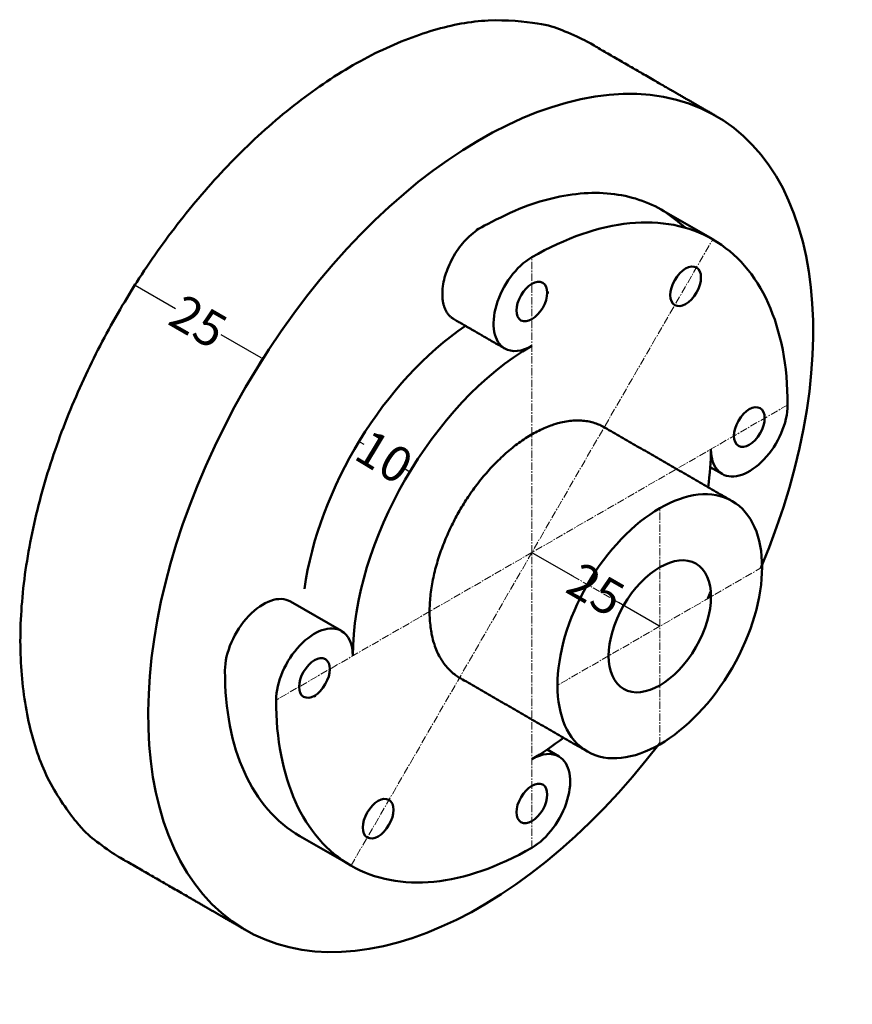
# Model space of a CAD drawing. Units: millimetres. Extents: x -66 to 75, y -3 to 164.
import ezdxf

# ---------------------------------------------------------------- set-up
doc = ezdxf.new("R2010")
doc.units = ezdxf.units.MM
doc.header["$MEASUREMENT"] = 0
doc.linetypes.add('CENTER', pattern=[2, 1.25, -0.25, 0.25, -0.25])
for name, color, linetype, lineweight in [('M-CNTR', 4, 'CENTER', 18), ('M-DIMS', 2, 'Continuous', 25), ('M-OUTL', 7, 'Continuous', 50)]:
    doc.layers.add(name, color=color, linetype=linetype, lineweight=lineweight)
doc.styles.get("Standard").update_dxf_attribs({"font": 'arial.ttf'})
doc.dimstyles.get("Standard").update_dxf_attribs({"dimtxt": 6, "dimasz": 0.18, "dimexe": 0.18, "dimexo": 0.0625, "dimgap": 0.09, "dimtad": 0, "dimtoh": 1, "dimdec": 0, "dimzin": 0, "dimdsep": 46, "dimtxsty": 'Standard', "dimcen": 0.09, "dimadec": 0, "dimazin": 0, "dimtfac": 1, "dimtdec": 0, "dimtofl": 0, "dimtmove": 0, "dimatfit": 3, "dimfxl": 1, "dimtolj": 1, "dimtzin": 0, "dimarcsym": 0})

# ---------------------------------------------------------------- blocks, each defined once
blk = doc.blocks.new('*D1')
at = {"layer": 'Defpoints', "color": 0, "transparency": 16777216}
for p in [(-49.36, 114.41), (-24.89, 106.8), (-27.71, 101.91)]:
    blk.add_point(p, dxfattribs=at)
at = {"layer": 'M-DIMS', "color": 0, "lineweight": -2, "transparency": 16777216}
for p, q in [((-49.33, 114.46), (-46.45, 119.45)), ((-46.38, 119.21), (-39.58, 115.28)), ((-25.05, 106.89), (-31.85, 110.82)), ((-27.68, 101.96), (-24.8, 106.95))]:
    blk.add_line(p, q, dxfattribs=at)
at = {"layer": 'M-DIMS', "color": 0, "transparency": 16777216}
for points in [[(-46.37, 119.23), (-46.4, 119.18), (-46.54, 119.3)], [(-25.03, 106.91), (-25.06, 106.86), (-24.89, 106.8)]]:
    blk.add_solid(points, dxfattribs=at)
at = {"layer": 'M-DIMS', "color": 0, "transparency": 16777216, "insert": (-35.71, 113.05), "char_height": 6, "attachment_point": 5, "rotation": 330}
blk.add_mtext('\\A1;25', dxfattribs=at)
blk = doc.blocks.new('*D2')
at = {"layer": 'Defpoints', "color": 0, "transparency": 16777216}
for p in [(-8.5, 92.73), (0.06, 87.56), (0.06, 87.56)]:
    blk.add_point(p, dxfattribs=at)
at = {"layer": 'M-DIMS', "color": 0, "lineweight": -2, "transparency": 16777216}
for p, q in [((-8.46, 92.78), (-8.4, 92.88)), ((-8.34, 92.63), (-7.72, 92.26)), ((-0.09, 87.65), (-0.71, 88.03)), ((0.1, 87.61), (0.16, 87.71))]:
    blk.add_line(p, q, dxfattribs=at)
at = {"layer": 'M-DIMS', "color": 0, "transparency": 16777216}
for points in [[(-8.33, 92.66), (-8.36, 92.61), (-8.5, 92.73)], [(-0.08, 87.68), (-0.11, 87.63), (0.06, 87.56)]]:
    blk.add_solid(points, dxfattribs=at)
at = {"layer": 'M-DIMS', "color": 0, "transparency": 16777216, "insert": (-4.22, 90.14), "char_height": 6, "attachment_point": 5, "rotation": 328.8743}
blk.add_mtext('\\A1;10', dxfattribs=at)
blk = doc.blocks.new('*D3')
at = {"layer": 'Defpoints', "color": 0, "transparency": 16777216}
for p in [(20.75, 73.93), (42.41, 61.43), (42.41, 61.43)]:
    blk.add_point(p, dxfattribs=at)
at = {"layer": 'M-DIMS', "color": 0, "lineweight": -2, "transparency": 16777216}
for p, q in [((20.79, 73.98), (20.84, 74.09)), ((20.91, 73.84), (27.72, 69.91)), ((42.25, 61.52), (35.44, 65.45)), ((42.44, 61.48), (42.5, 61.59))]:
    blk.add_line(p, q, dxfattribs=at)
at = {"layer": 'M-DIMS', "color": 0, "transparency": 16777216}
for points in [[(20.93, 73.87), (20.9, 73.81), (20.75, 73.93)], [(42.26, 61.55), (42.23, 61.49), (42.41, 61.43)]]:
    blk.add_solid(points, dxfattribs=at)
at = {"layer": 'M-DIMS', "color": 0, "transparency": 16777216, "insert": (31.58, 67.68), "char_height": 6, "attachment_point": 5, "rotation": 330}
blk.add_mtext('\\A1;25', dxfattribs=at)

msp = doc.modelspace()

# ---------------------------------------------------------------- linework, layer by layer
at = {"layer": 'M-CNTR'}
for p, q in [((-9.86, 20.9), (51.37, 126.96)), ((20.75, 23.93), (20.75, 123.93)), ((64.06, 98.93), (-22.55, 48.93)), ((42.41, 41.43), (42.41, 81.43)), ((20.75, 73.93), (42.41, 61.43)), ((59.73, 71.43), (25.08, 51.43))]:
    msp.add_line(p, q, dxfattribs=at)
at = {"layer": 'M-OUTL'}
for p, q in [((42.71, 131.97), (51.37, 126.97)), ((50.96, 88.39), (52.97, 87.23)), ((-20.12, 65.64), (-11.46, 60.64)), ((23.33, 40.55), (25.35, 39.39)), ((-18.52, 25.9), (-9.86, 20.9))]:
    msp.add_line(p, q, dxfattribs=at)
for centre, major_axis, start_param, end_param in [((12.09, 78.93), (-39.8, -68.94), 1.787584, 7.637194), ((20.75, 73.93), (-30.62, -53.03), 3.141593, 3.926988), ((-9.56, 91.43), (-39.8, -68.94), 2.435548, 2.437589), ((20.75, 73.93), (-30.62, -53.03), 2.356197, 3.141593), ((20.75, 116.43), (-4.59, -7.95), 3.926991, 6.283185), ((12.09, 78.93), (-21.43, -37.12), 3.536931, 3.546444), ((12.09, 78.93), (-21.43, -37.12), 4.012224, 5.323526), ((20.75, 73.93), (21.43, 37.12), 0.785398, 2.356194), ((20.75, 116.43), (-4.59, -7.95), 0, 0.785398), ((57.56, 95.18), (-4.59, -7.95), 0, 2.356194), ((20.75, 73.93), (21.43, 37.12), 5.320635, 5.497787), ((57.56, 95.18), (-4.59, -7.95), 5.497787, 6.283185), ((-24.71, 57.68), (-4.59, -7.95), 3.141593, 5.497787), ((20.75, 73.93), (-26.03, -45.08), 8.010505, 8.034725), ((-16.05, 52.68), (-4.59, -7.95), 3.141593, 5.497787), ((-16.05, 52.68), (-4.59, -7.95), 2.356194, 3.141593), ((12.09, 78.93), (-30.62, -53.03), 5.49779, 6.283185), ((20.75, 73.93), (-30.62, -53.03), 5.49779, 6.283185), ((12.09, 78.93), (-21.43, -37.12), 5.878334, 5.887847), ((20.75, 73.93), (21.43, 37.12), 3.926991, 4.104143), ((20.75, 31.43), (-4.59, -7.95), 3.141593, 3.926991), ((20.75, 31.43), (-4.59, -7.95), 0.785398, 3.141593), ((20.75, 73.93), (-30.62, -53.03), 0, 0.785395)]:
    msp.add_ellipse(centre, major_axis=major_axis, ratio=0.57735, start_param=start_param, end_param=end_param, dxfattribs=at)
for centre, major_axis in [((46.78, 119.01), (-1.84, -3.18)), ((20.75, 116.43), (-1.84, -3.18)), ((57.56, 95.18), (-1.84, -3.18)), ((42.41, 61.43), (-12.25, -21.21)), ((42.41, 61.43), (-6.12, -10.61)), ((-16.05, 52.68), (-1.84, -3.18)), ((20.75, 31.43), (-1.84, -3.18)), ((-5.27, 28.85), (-1.84, -3.18))]:
    msp.add_ellipse(centre, major_axis=major_axis, ratio=0.57735, dxfattribs=at)
for points, weights, knots in [([(51.9, 147.87), (41.07, 154.12), (30.25, 160.37), (-9.56, 183.35), (-49.36, 114.41), (-89.16, 45.47), (-49.36, 22.49), (-38.54, 16.24), (-27.71, 9.99)], [1, 1, 1, 0.707106781187, 1, 0.707106781187, 1, 1, 1], [0, 0, 0, 1, 1, 2.570796, 2.570796, 4.141593, 4.141593, 5.141593, 5.141593, 5.141593]), ([(46.74, 128.93), (33.75, 141.43), (12.09, 128.93), (7.75, 126.42), (6.09, 120.84), (4.43, 115.25), (7.5, 113.47), (11.83, 110.97), (16.16, 108.47)], [1, 0.894427191, 1, 0.831469612303, 1, 0.831469612303, 1, 1, 1], [0, 0, 0, 0.927295, 0.927295, 2.105392, 2.105392, 3.28349, 3.28349, 4.28349, 4.28349, 4.28349]), ([(54.65, 82.64), (43.83, 88.89), (33, 95.14), (20.75, 102.21), (8.51, 81), (-3.74, 59.79), (8.51, 52.72), (19.33, 46.47), (30.16, 40.22)], [1, 1, 1, 0.707106781187, 1, 0.707106781187, 1, 1, 1], [0, 0, 0, 1, 1, 2.570796, 2.570796, 4.141593, 4.141593, 5.141593, 5.141593, 5.141593])]:
    msp.add_rational_spline(points, weights, degree=2, knots=knots, dxfattribs=at)

# ---------------------------------------------------------------- dimensions: what is measured, and where the dimension line sits
at = {"layer": 'M-DIMS'}
for p1, p2, distance, picture, middle in [((-49.36, 114.41), (-27.71, 101.91), 5.64, '*D1', (-35.71, 113.05)), ((-8.5, 92.73), (0.06, 87.56), 0, '*D2', (-4.22, 90.14)), ((20.75, 73.93), (42.41, 61.43), 0, '*D3', (31.58, 67.68))]:
    dim = msp.add_aligned_dim(p1=p1, p2=p2, distance=distance, dimstyle='Standard', override={"dimclrd": 0, "dimclre": 0, "dimclrt": 0}, dxfattribs=at)
    dim.commit()
    dim.dimension.update_dxf_attribs({"geometry": picture, "text_midpoint": middle})

doc.saveas('drawing.dxf')
